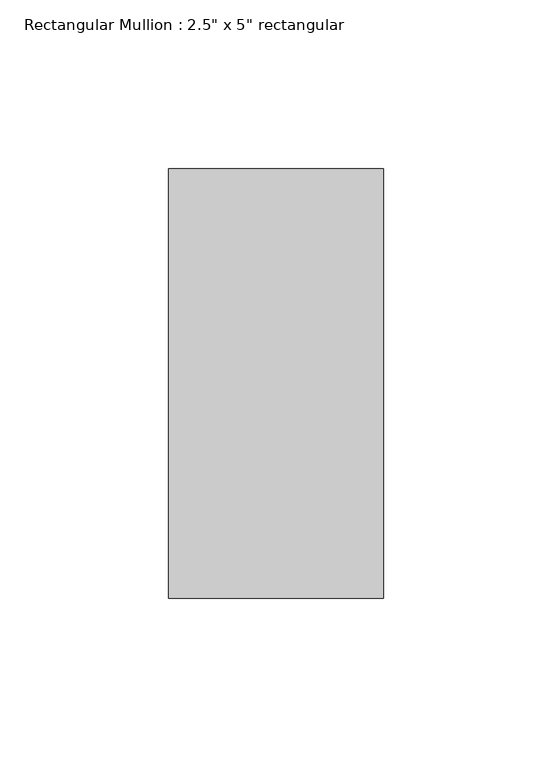
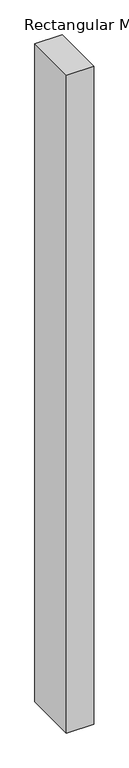
"""IFC4 building model written with IfcOpenShell, lengths in millimetres: member geometry."""

from ifc_helpers import new_model, si_unit, frame, origin, place, context, project, spatial, polyline, outline, extrude, source, transform, mapped, element, save


def member_8456be0a(model_context):
    return source(origin(), model_context, "Body", "SweptSolid", [
        extrude(outline(polyline([(31.75, 63.5), (31.75, -63.5), (-31.75, -63.5), (-31.75, 63.5), (31.75, 63.5)])), frame((0.0, 0.0, -1619.7840707), z_axis=(0.0, 0.0, 1.0), x_axis=(1.0, 0.0, 0.0)), (0.0, 0.0, 1.0), 1619.7840707),
    ])


if __name__ == "__main__":
    model = new_model("IFC4")
    model_context = context("Model", 3, world=origin())
    ifc_project = project(units=[si_unit("LENGTHUNIT", "METRE", prefix="MILLI")], contexts=[model_context])
    site = spatial("IfcSite", under=ifc_project)
    building = spatial("IfcBuilding", under=site)
    placement = place(None, origin())
    member_shape = member_8456be0a(model_context)
    element("IfcMember", 1, ObjectType="Rectangular Mullion : 2.5\" x 5\" rectangular", at=placement, inside=building, context=model_context, shape_type="MappedRepresentation", body=[
        mapped(member_shape, transform((0.0, 0.0, 0.0), x_axis=(1.0, 0.0, 0.0), y_axis=(0.0, 1.0, 0.0), z_axis=(0.0, 0.0, 1.0))),
    ])
    save(model, "model.ifc")

# Revit data of these elements
# Type "Rectangular Mullion : 2.5\" x 5\" rectangular"
#   built-in parameter 1007304 = 0.416667 (stored number, unit not read)
#   built-in parameter 1007301 = 0.104167 (stored number, unit not read)
#   built-in parameter 1007300 = 0.104167 (stored number, unit not read)
# Element 1 (IfcMember, "Rectangular Mullion : 2.5\" x 5\" rectangular")
#   Materials on its faces: "Aluminum"
# Materials
#   "Aluminum": class "Metal", colour RGB 247 247 247, transparency 0, Description = "Aluminum 6061", Cost = 0
